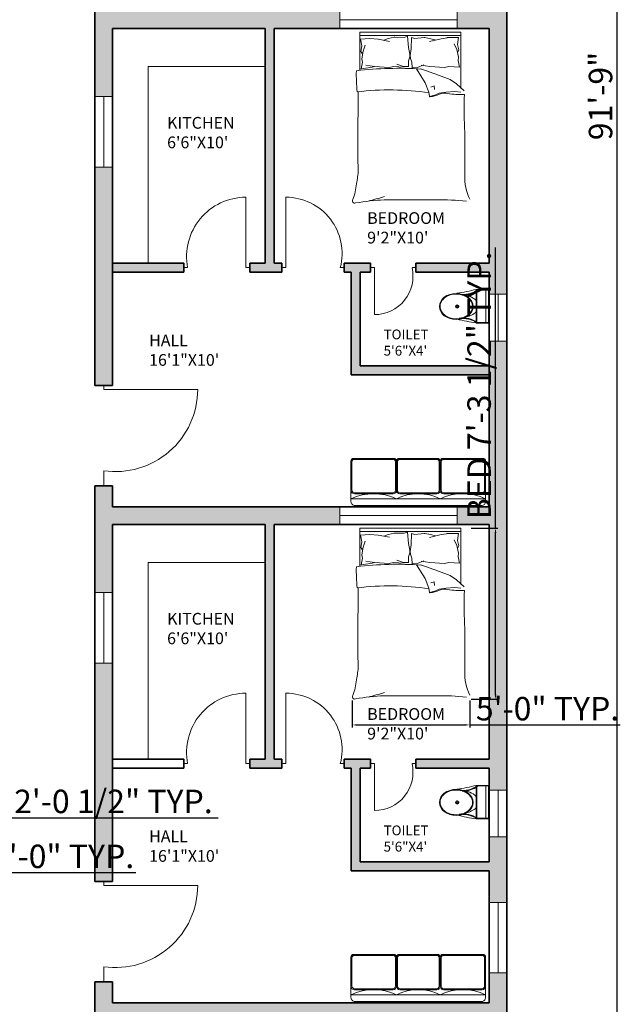
# Model space of a CAD drawing. Units: inches. Extents: x 1266 to 2869, y -408 to 3241.
# Tile 3 of 11: x 1710 to 2017, y 1264 to 1767. Entities that reach past the tile are written whole.
import ezdxf

# ---------------------------------------------------------------- set-up
doc = ezdxf.new("R2010")
doc.units = ezdxf.units.IN
for name, color, linetype, lineweight in [('A-ANNO-DIMS', 2, 'Continuous', 18), ('A-AREA-IDEN', 7, 'Continuous', 18), ('A-DOOR', 4, 'Continuous', 18), ('A-FLOR-CASE', 9, 'Continuous', 18), ('A-FLOR-FIXT', 9, 'Continuous', 18), ('A-FURN', 8, 'Continuous', 18), ('A-GLAZ', 4, 'Continuous', 18), ('A-WALL', 7, 'Continuous', 35), ('A-WALL-PATT', 251, 'Continuous', 13)]:
    doc.layers.add(name, color=color, linetype=linetype, lineweight=lineweight)
doc.styles.get("Standard").update_dxf_attribs({"font": 'arial.ttf'})
doc.dimstyles.new('ISO-25', dxfattribs={"dimtxt": 12, "dimasz": 2.5, "dimexe": 1.25, "dimexo": 0.625, "dimtad": 1, "dimdec": 0, "dimlunit": 3, "dimtxsty": 'Standard', "dimcen": 2.5, "dimadec": 0, "dimazin": 0, "dimtfac": 1, "dimtdec": 0, "dimtmove": 0, "dimatfit": 3, "dimfxl": 1, "dimarcsym": 0})

# ---------------------------------------------------------------- blocks, each defined once
blk = doc.blocks.new('A$C31115884')
for p, q in [((283, 498), (223, 498)), ((258, 466), (258, 523)), ((0, 200), (0, 0)), ((520, 200), (0, 200)), ((10, 190), (10, 10)), ((510, 190), (10, 190)), ((510, 10), (510, 190)), ((520, 0), (520, 200)), ((510, 54), (0, 54)), ((10, 10), (510, 10)), ((0, 0), (520, 0))]:
    blk.add_line(p, q)
blk.add_circle((256, 496), 23.6)
for centre, radius, start, end in [((2778, -205), 2807, 165.4549, 171.7133), ((-295, 403), 365, 324.2091, 9.3499), ((-295, 403), 375, 324.2091, 9.3499), ((806, 403), 365, 170.6501, 215.7909), ((3237, 905), 2807, 188.2867, 194.5451), ((384, 406), 293, 190.2774, 224.1564), ((139, 406), 293, 315.8436, 2.6563), ((806, 403), 375, 179.2036, 215.7909)]:
    blk.add_arc(centre, radius, start, end)
blk.add_ellipse((256, 510), major_axis=(0, -261), ratio=0.772727)
blk.add_open_spline([(256, 259), (263, 259), (270, 260), (288, 262), (299, 265), (320, 273), (330, 278), (350, 291), (360, 299), (378, 316), (386, 326), (402, 347), (409, 358), (421, 383), (427, 395), (436, 422), (440, 436), (445, 465), (447, 480), (448, 509), (448, 524), (445, 553), (443, 568), (436, 596), (432, 610), (422, 636), (416, 649), (402, 672), (395, 683), (379, 703), (370, 712), (351, 728), (341, 735), (321, 746), (310, 751), (289, 757), (278, 759), (256, 761), (245, 761), (223, 757), (212, 754), (191, 746), (181, 741), (161, 728), (151, 720), (133, 703), (125, 693), (110, 672), (103, 660), (90, 636), (85, 623), (76, 596), (72, 582), (67, 553), (66, 538), (64, 509), (65, 494), (68, 465), (70, 450), (77, 422), (81, 408), (91, 382), (97, 370), (111, 346), (118, 335), (135, 316), (144, 307), (162, 291), (172, 284), (193, 273), (203, 269), (225, 262), (236, 260), (250, 259), (253, 259), (256, 259)], degree=3, knots=[0, 0, 0, 0, 0.110105, 0.110105, 0.285049, 0.285049, 0.459994, 0.459994, 0.634938, 0.634938, 0.809882, 0.809882, 0.984827, 0.984827, 1.159771, 1.159771, 1.334715, 1.334715, 1.50966, 1.50966, 1.684604, 1.684604, 1.859549, 1.859549, 2.034493, 2.034493, 2.209437, 2.209437, 2.384382, 2.384382, 2.559326, 2.559326, 2.73427, 2.73427, 2.909215, 2.909215, 3.084159, 3.084159, 3.259103, 3.259103, 3.434048, 3.434048, 3.608992, 3.608992, 3.783936, 3.783936, 3.958881, 3.958881, 4.133825, 4.133825, 4.30877, 4.30877, 4.483714, 4.483714, 4.658658, 4.658658, 4.833603, 4.833603, 5.008547, 5.008547, 5.183491, 5.183491, 5.358436, 5.358436, 5.53338, 5.53338, 5.708324, 5.708324, 5.883269, 5.883269, 6.058213, 6.058213, 6.233158, 6.233158, 6.283185, 6.283185, 6.283185, 6.283185])
blk = doc.blocks.new('*D3')
at = {"layer": 'A-ANNO-DIMS', "color": 0, "lineweight": -2, "transparency": 16777216}
for p, q in [((1959.32, 2278.35), (2016.1, 2278.35)), ((2014.85, 2275.85), (2014.85, 1179.85)), ((1959.32, 1177.35), (2016.1, 1177.35))]:
    blk.add_line(p, q, dxfattribs=at)
at = {"layer": 'A-ANNO-DIMS', "color": 0, "transparency": 16777216}
for points in [[(2014.43, 2275.85), (2015.27, 2275.85), (2014.85, 2278.35)], [(2014.43, 1179.85), (2015.27, 1179.85), (2014.85, 1177.35)]]:
    blk.add_solid(points, dxfattribs=at)
at = {"layer": 'Defpoints', "color": 0, "transparency": 16777216}
for p in [(1958.69, 2278.35), (1958.69, 1177.35), (2014.85, 1177.35)]:
    blk.add_point(p, dxfattribs=at)
at = {"layer": 'A-ANNO-DIMS', "color": 0, "transparency": 16777216, "insert": (2008.1, 1727.85), "char_height": 12, "attachment_point": 5, "rotation": 90}
blk.add_mtext('91\'-9"', dxfattribs=at)
blk = doc.blocks.new('BED-DOUBLE-2')
for p, q in [((3.76, 67.77), (3.76, 87.35)), ((3.76, 87.35), (55.42, 87.35)), ((3.76, 85.69), (55.42, 85.69)), ((55.42, 87.35), (55.42, 58.59)), ((4.21, 83.74), (8.84, 84.1)), ((4.21, 83.77), (4.84, 80.33)), ((5.46, 77.67), (6.55, 80.64)), ((8.84, 84.1), (8.96, 84.08)), ((8.96, 84.08), (13.09, 83.77)), ((13.09, 83.77), (19.03, 82.67)), ((16.06, 83.3), (18.25, 84.08)), ((18.25, 84.08), (21.37, 84.86)), ((21.37, 84.86), (21.72, 84.86)), ((21.72, 84.86), (26.53, 84.7)), ((26.53, 84.7), (28.09, 85.33)), ((28.09, 85.33), (28.71, 79.55)), ((30.24, 84.66), (29.98, 78.85)), ((31.84, 84.13), (30.24, 84.66)), ((36.63, 84.59), (31.84, 84.13)), ((36.98, 84.61), (36.63, 84.59)), ((40.14, 84.02), (36.98, 84.61)), ((45.31, 84.03), (39.45, 82.57)), ((42.38, 83.38), (40.14, 84.02)), ((49.42, 84.6), (45.31, 84.03)), ((54.17, 84.59), (48.33, 84.69)), ((48.33, 84.69), (49.42, 84.6)), ((53.31, 78.43), (52.03, 81.32)), ((54.17, 84.59), (53.76, 81.12)), ((53.76, 81.12), (54.41, 78.34)), ((4.84, 80.33), (4.37, 77.51)), ((4.37, 77.51), (4.99, 76.42)), ((4.84, 73.76), (5.46, 77.67)), ((28.71, 79.55), (29.34, 76.11)), ((29.34, 76.11), (29.34, 74.7)), ((29.98, 78.85), (29.57, 75.38)), ((54.17, 74.56), (53.31, 78.43)), ((54.41, 78.34), (53.85, 77.21)), ((4.52, 68.61), (5.15, 72.04)), ((5.15, 72.04), (4.84, 73.76)), ((26.06, 69.77), (22.66, 70.95)), ((29.34, 74.7), (28.71, 72.67)), ((28.71, 72.67), (28.71, 69.77)), ((29.57, 75.38), (29.66, 73.97)), ((29.66, 73.97), (30.41, 71.98)), ((30.41, 71.98), (30.59, 69.09)), ((33.24, 69.26), (36.56, 70.64)), ((53.97, 72.83), (54.17, 74.56)), ((54.81, 69.44), (53.97, 72.83)), ((10.03, 69.39), (4.52, 68.61)), ((6.9, 70.46), (11.26, 69.74)), ((11.26, 69.74), (10.03, 69.39)), ((11.26, 69.74), (18.84, 69.27)), ((18.84, 69.27), (20.95, 69.87)), ((20.95, 69.87), (26.5, 69.44)), ((28.71, 69.77), (26.06, 69.77)), ((30.59, 69.09), (33.24, 69.26)), ((32.71, 68.56), (37.24, 61.54)), ((43.94, 65.39), (34.92, 68.56)), ((35.2, 70.46), (39.56, 69.74)), ((39.56, 69.74), (47.14, 69.27)), ((47.14, 69.27), (49.26, 69.87)), ((49.26, 69.87), (54.81, 69.44)), ((37.24, 61.54), (39.08, 56.69)), ((49.96, 63.21), (43.94, 65.39)), ((53.15, 60.87), (49.96, 63.21)), ((57.15, 57.36), (53.15, 60.87)), ((39.08, 56.69), (39.42, 54.51)), ((40.12, 59.32), (41.78, 59.99)), ((41.87, 58.1), (41.78, 59.99, 4.18)), ((42.1, 55.18), (44.27, 56.19)), ((44.27, 56.19), (47.96, 56.69)), ((47.96, 56.69), (52.14, 57.02)), ((52.14, 57.02), (55.49, 56.69)), ((39.42, 54.51), (42.1, 55.18)), ((16.28, 1.69), (42.89, 1.69))]:
    blk.add_line(p, q)
for centre, radius, start, end in [((92.06, 65.63), 90.06, 178.7218, 185.604), ((23.09, -109.45), 178.34, 86.0865, 96.7821), ((19.19, -81.63), 139.47, 81.7845, 96.9006), ((-180.86, 53.65), 183.89, 358.4762, 1.0082), ((33.68, 85.75), 32.06, 280.6617, 289.8806), ((47.29, 49.44), 6.73, 78.6608, 113.7384), ((55.49, 94.55), 39.11, 259.8763, 272.5657), ((197.03, 48.09), 139.99, 176.9791, 183.8365), ((39.61, 54.45), 0.199, 160.2464, 271.1377), ((524.11, 32.64), 521.39, 178.2277, 181.7185), ((-4874.07, 14.03), 4931.49, 0.00217, 0.28689), ((-29.08, 17.61), 32.04, 346.0648, 358.9113), ((82.33, 13.12), 24.93, 177.4714, 206.4681), ((-23.41, 11.38), 25.47, 337.9751, 356.652), ((1.18, 1.17), 1.18, 146.1736, 293.4781), ((23.16, -129.76), 131.62, 92.9958, 99.4091), ((-18.62, 112.98), 115.08, 283.3832, 287.7053), ((44.49, -142.12), 143.82, 84.4998, 90.6351)]:
    blk.add_arc(centre, radius, start, end)
blk = doc.blocks.new('SOFA-3-SEAT')
for points in [[(0, 22.36), (0, 7.74, 0.414214), (1.72, 6.02), (21.5, 6.02, 0.414214), (23.22, 7.74), (23.22, 22.36, 0.414214), (21.5, 24.08), (1.72, 24.08, 0.414214)], [(0.52, 22.36), (0.52, 7.74, 0.414214), (1.72, 6.54), (21.5, 6.54, 0.414214), (22.7, 7.74), (22.7, 22.36, 0.414214), (21.5, 23.56), (1.72, 23.56, 0.414214)], [(45.57, 22.36), (45.57, 7.74, -0.414214), (43.85, 6.02), (24.94, 6.02, -0.414214), (23.22, 7.74), (23.22, 22.36, -0.414214), (24.94, 24.08), (43.85, 24.08, -0.414214)], [(45.06, 22.36), (45.06, 7.74, -0.414214), (43.85, 6.54), (24.94, 6.54, -0.414214), (23.73, 7.74), (23.73, 22.36, -0.414214), (24.94, 23.56), (43.85, 23.56, -0.414214)], [(45.57, 22.36), (45.57, 7.74, 0.414214), (47.29, 6.02), (67.07, 6.02, 0.414214), (68.79, 7.74), (68.79, 22.36, 0.414214), (67.07, 24.08), (47.29, 24.08, 0.414214)], [(46.09, 22.36), (46.09, 7.74, 0.414214), (47.29, 6.54), (67.07, 6.54, 0.414214), (68.27, 7.74), (68.27, 22.36, 0.414214), (67.07, 23.56), (47.29, 23.56, 0.414214)]]:
    blk.add_lwpolyline(points, format="xyb", close=True)
at = {"ltscale": 0.03}
blk.add_lwpolyline([(21.82, 24.08), (1.38, 24.08, 0.414214), (0, 22.7), (0, 2.06, 0.414214), (2.06, 0), (66.73, 0, 0.414214), (68.79, 2.06), (68.79, 22.7, 0.414214), (67.41, 24.08), (46.97, 24.08, 0.414214), (45.59, 22.7, -1), (45.56, 22.7, 0.414214), (44.18, 24.08), (24.61, 24.08, 0.414214), (23.23, 22.7, -1), (23.2, 22.7, 0.414214)], format="xyb", close=True, dxfattribs=at)
blk.add_lwpolyline([(0, 3.44), (68.79, 3.44)])
for centre, radius, start, end in [((11.61, -21.35), 27.38, 64.9106, 115.0894), ((34.4, -19.35), 25.38, 63.869, 116.131), ((57.18, -21.07), 27.12, 64.6538, 115.3462)]:
    blk.add_arc(centre, radius, start, end)
blk = doc.blocks.new('DOOR-KITCHEN-R')
for p, q in [((31.78, 0), (31.78, 36)), ((0, 0), (2, 0)), ((33.78, 0), (31.78, 0))]:
    blk.add_line(p, q)
blk.add_arc((31.78, 5.68), 30.32, 90, 190.7956)
blk = doc.blocks.new('DOOR-BEDROOM-R')
for p, q in [((2, 0), (2, 36)), ((0, 0), (2, 0)), ((31.84, 0), (29.84, 0))]:
    blk.add_line(p, q)
blk.add_arc((2, 7.24), 28.76, 345.4318, 90)
blk = doc.blocks.new('DOOR-BATH-R')
for p, q in [((0, 24), (2, 24)), ((2, 24), (2, 0)), ((23.14, 24), (21.14, 24))]:
    blk.add_line(p, q)
blk.add_arc((2, 19.63), 19.63, 270, 12.8499)
blk = doc.blocks.new('DOOR-ENTRY-R')
for p, q in [((0, 51.27), (0, 49.27)), ((0, 49.27), (36, 49.27)), ((36, 49.27), (48, 49.27)), ((0, 5.68), (0, 7.68)), ((0, 0), (0, 5.68))]:
    blk.add_line(p, q)
blk.add_arc((5.98, 49.27), 42.02, 261.8116, 0)
blk = doc.blocks.new('WIN-PLAN-60')
for p, q in [((0, 9), (0, 0)), ((60, 4.5), (60, 9)), ((60, 9), (60, 0)), ((0, 4.5), (60, 4.5)), ((0, 0), (0, 4.5))]:
    blk.add_line(p, q)
blk = doc.blocks.new('WIN-PLAN-36')
for p, q in [((0, 36), (9, 36)), ((4.5, 36), (4.5, 0)), ((9, 36), (4.5, 36)), ((4.5, 0), (0, 0)), ((0, 0), (9, 0))]:
    blk.add_line(p, q)
blk = doc.blocks.new('WIN-PLAN-24')
for p, q in [((0, 24), (9, 24)), ((4.5, 24), (4.5, 0)), ((9, 24), (4.5, 24)), ((0, 0), (9, 0))]:
    blk.add_line(p, q)
blk = doc.blocks.new('COUNTER-KITCHEN')
for p, q in [((0, 0), (0, 100.54)), ((0, 100.54), (59.82, 100.54))]:
    blk.add_line(p, q)
blk = doc.blocks.new('*D35')
at = {"layer": 'A-ANNO-DIMS', "color": 0, "lineweight": -2, "transparency": 16777216}
for p, q in [((1627.24, 1361.97), (1627.24, 1357.64)), ((1629.74, 1358.89), (1649.44, 1358.89)), ((1651.94, 1361.97), (1651.94, 1357.64)), ((1651.94, 1358.89), (1811.15, 1358.89))]:
    blk.add_line(p, q, dxfattribs=at)
at = {"layer": 'A-ANNO-DIMS', "color": 0, "transparency": 16777216}
for points in [[(1629.74, 1359.31), (1629.74, 1358.48), (1627.24, 1358.89)], [(1649.44, 1359.31), (1649.44, 1358.48), (1651.94, 1358.89)]]:
    blk.add_solid(points, dxfattribs=at)
at = {"layer": 'Defpoints', "color": 0, "transparency": 16777216}
for p in [(1627.24, 1362.6), (1651.94, 1362.6), (1651.94, 1358.89)]:
    blk.add_point(p, dxfattribs=at)
at = {"layer": 'A-ANNO-DIMS', "color": 0, "transparency": 16777216, "insert": (1732.8, 1365.73), "char_height": 12, "attachment_point": 5}
blk.add_mtext('DOOR 2\'-0 1/2" TYP.', dxfattribs=at)
blk = doc.blocks.new('*D41')
at = {"layer": 'A-ANNO-DIMS', "color": 0, "lineweight": -2, "transparency": 16777216}
for p, q in [((1952.88, 1506.96), (1952.88, 1650.41)), ((1940.39, 1506.96), (1954.13, 1506.96)), ((1952.88, 1421.99), (1952.88, 1504.46)), ((1940.39, 1419.49), (1954.13, 1419.49))]:
    blk.add_line(p, q, dxfattribs=at)
at = {"layer": 'A-ANNO-DIMS', "color": 0, "transparency": 16777216}
for points in [[(1952.46, 1504.46), (1953.3, 1504.46), (1952.88, 1506.96)], [(1952.46, 1421.99), (1953.3, 1421.99), (1952.88, 1419.49)]]:
    blk.add_solid(points, dxfattribs=at)
at = {"layer": 'Defpoints', "color": 0, "transparency": 16777216}
for p in [(1939.76, 1506.96), (1952.88, 1506.96), (1939.76, 1419.49)]:
    blk.add_point(p, dxfattribs=at)
at = {"layer": 'A-ANNO-DIMS', "color": 0, "transparency": 16777216, "insert": (1946.05, 1579.94), "char_height": 12, "attachment_point": 5, "rotation": 90}
blk.add_mtext('BED 7\'-3 1/2" TYP.', dxfattribs=at)
blk = doc.blocks.new('*D42')
at = {"layer": 'A-ANNO-DIMS', "color": 0, "lineweight": -2, "transparency": 16777216}
for p, q in [((1879.66, 1418.87), (1879.66, 1405.12)), ((1939.76, 1418.87), (1939.76, 1405.12)), ((1882.16, 1406.37), (1937.26, 1406.37)), ((1939.76, 1406.37), (2016.66, 1406.37))]:
    blk.add_line(p, q, dxfattribs=at)
at = {"layer": 'A-ANNO-DIMS', "color": 0, "transparency": 16777216}
for points in [[(1882.16, 1406.79), (1882.16, 1405.96), (1879.66, 1406.37)], [(1937.26, 1406.79), (1937.26, 1405.96), (1939.76, 1406.37)]]:
    blk.add_solid(points, dxfattribs=at)
at = {"layer": 'Defpoints', "color": 0, "transparency": 16777216}
for p in [(1879.66, 1419.49), (1939.76, 1419.49), (1939.76, 1406.37)]:
    blk.add_point(p, dxfattribs=at)
at = {"layer": 'A-ANNO-DIMS', "color": 0, "transparency": 16777216, "insert": (1979.46, 1413.13), "char_height": 12, "attachment_point": 5}
blk.add_mtext('5\'-0" TYP.', dxfattribs=at)
blk = doc.blocks.new('*D46')
at = {"layer": 'A-ANNO-DIMS', "color": 0, "lineweight": -2, "transparency": 16777216}
for p, q in [((1643.69, 1323.83), (1643.69, 1332.15)), ((1646.19, 1330.9), (1689.19, 1330.9)), ((1691.69, 1323.83), (1691.69, 1332.15)), ((1691.69, 1330.9), (1769.07, 1330.9))]:
    blk.add_line(p, q, dxfattribs=at)
at = {"layer": 'A-ANNO-DIMS', "color": 0, "transparency": 16777216}
for points in [[(1646.19, 1331.32), (1646.19, 1330.48), (1643.69, 1330.9)], [(1689.19, 1331.32), (1689.19, 1330.48), (1691.69, 1330.9)]]:
    blk.add_solid(points, dxfattribs=at)
at = {"layer": 'Defpoints', "color": 0, "transparency": 16777216}
for p in [(1691.69, 1330.9), (1643.69, 1323.21), (1691.69, 1323.21)]:
    blk.add_point(p, dxfattribs=at)
at = {"layer": 'A-ANNO-DIMS', "color": 0, "transparency": 16777216, "insert": (1731.63, 1337.65), "char_height": 12, "attachment_point": 5}
blk.add_mtext('4\'-0" TYP.', dxfattribs=at)

msp = doc.modelspace()

# ---------------------------------------------------------------- hatches: boundary and pattern name
at = {"layer": 'A-WALL-PATT'}
h = msp.add_hatch(color=256, dxfattribs=at)
h.dxf.hatch_style = 1
h.paths.add_polyline_path([(1484.69, 2269.35), (1562.69, 2269.35), (1562.69, 2149.35), (1558.42, 2149.35), (1558.42, 2144.85), (1567.19, 2144.85), (1573.23, 2144.85), (1573.23, 2146.74), (1573.23, 2149.35), (1567.19, 2149.35), (1567.19, 2269.35), (1597.45, 2269.35), (1597.45, 2273.85), (1597.45, 2278.35), (1475.69, 2278.35), (1475.69, 2234.52), (1484.69, 2234.52)])
h.paths.add_polyline_path([(1873.25, 2278.35), (1748.19, 2278.35), (1696.19, 2278.35), (1657.45, 2278.35), (1657.45, 2269.35), (1687.19, 2269.35), (1687.19, 2149.35), (1651.94, 2149.35), (1651.94, 2144.85), (1687.19, 2144.85), (1687.19, 2133.61), (1696.19, 2133.61), (1696.19, 2269.35), (1748.19, 2269.35), (1748.19, 2234.52), (1757.19, 2234.52), (1757.19, 2269.35), (1835.19, 2269.35), (1835.19, 2149.35), (1827.33, 2149.35), (1827.33, 2144.85), (1843.74, 2144.85), (1843.74, 2149.35), (1839.69, 2149.35), (1839.69, 2269.35), (1873.25, 2269.35), (1873.25, 2273.85)])
h.paths.add_polyline_path([(1958.69, 2278.35), (1933.25, 2278.35), (1933.25, 2269.35), (1949.69, 2269.35), (1949.69, 2149.35), (1912.22, 2149.35), (1912.22, 2144.85), (1949.69, 2144.85), (1949.69, 2133.61), (1958.69, 2133.61)])
h.paths.add_polyline_path([(1883.69, 2144.85), (1889.08, 2144.85), (1889.08, 2149.35), (1875.58, 2149.35), (1875.58, 2144.85), (1879.19, 2144.85), (1879.19, 2092.35), (1949.69, 2092.35), (1949.69, 2086.89), (1949.69, 2024.85), (1933.25, 2024.85), (1933.25, 2015.85), (1949.69, 2015.85), (1949.69, 1895.85), (1912.45, 1895.85), (1912.45, 1891.35), (1949.69, 1891.35), (1949.69, 1880.11), (1958.69, 1880.11), (1958.69, 2086.89), (1958.69, 2109.61), (1949.69, 2109.61), (1949.69, 2096.85), (1883.69, 2096.85)])
h.paths.add_polyline_path([(1757.19, 2198.52), (1748.19, 2198.52), (1748.19, 2086.89), (1757.19, 2086.89), (1757.19, 2144.85), (1793.55, 2144.85), (1793.55, 2149.35), (1757.19, 2149.35)])
h.paths.add_polyline_path([(1696.19, 2109.61), (1687.19, 2109.61), (1687.19, 2096.85), (1621.19, 2096.85), (1621.19, 2144.85), (1627.24, 2144.85), (1627.24, 2149.35), (1616.69, 2149.35), (1610.35, 2149.35), (1610.35, 2144.85), (1616.69, 2144.85), (1616.69, 2092.35), (1687.19, 2092.35), (1687.19, 2086.89), (1696.19, 2086.89)], flags=17)
h.paths.add_polyline_path([(1484.69, 2144.85), (1520.8, 2144.85), (1520.8, 2149.35), (1484.69, 2149.35), (1484.69, 2198.52), (1475.69, 2198.52), (1475.69, 1981.02), (1484.69, 1981.02), (1484.69, 2015.85), (1687.19, 2015.85), (1687.19, 1895.85), (1650.13, 1895.85), (1650.13, 1891.35), (1687.19, 1891.35), (1687.19, 1880.11), (1696.19, 1880.11), (1696.19, 2035.62), (1687.19, 2035.62), (1687.19, 2024.85), (1484.69, 2024.85)])
h.paths.add_polyline_path([(1484.69, 1691.52), (1475.69, 1691.52), (1475.69, 1474.02), (1484.69, 1474.02)])
h.paths.add_polyline_path([(1518.03, 1895.85), (1484.69, 1895.85), (1484.69, 1945.02), (1475.69, 1945.02), (1475.69, 1727.52), (1484.69, 1727.52), (1484.69, 1762.35), (1687.19, 1762.35), (1687.19, 1642.35), (1651.94, 1642.35), (1651.94, 1637.85), (1687.19, 1637.85), (1687.19, 1589.85), (1621.19, 1589.85), (1621.19, 1637.85), (1627.19, 1637.85), (1627.19, 1642.35), (1610.89, 1642.35), (1610.89, 1637.85), (1616.69, 1637.85), (1616.69, 1585.35), (1687.19, 1585.35), (1687.19, 1579.45), (1696.19, 1579.45), (1696.19, 1779.84), (1687.19, 1779.84), (1687.19, 1771.35), (1484.69, 1771.35), (1484.69, 1891.35), (1518.03, 1891.35)])
h.paths.add_polyline_path([(1567.19, 2015.85), (1562.69, 2015.85), (1562.69, 1895.85), (1555.64, 1895.85), (1555.64, 1891.35), (1570.46, 1891.35), (1570.46, 1895.85), (1567.19, 1895.85)], flags=17)
h.paths.add_polyline_path([(1625.43, 1895.85), (1607.58, 1895.85), (1607.58, 1891.35), (1616.69, 1891.35), (1616.69, 1838.85), (1687.19, 1838.85), (1687.19, 1831.11), (1696.19, 1831.11), (1696.19, 1856.11), (1687.19, 1856.11), (1687.19, 1843.35), (1621.19, 1843.35), (1621.19, 1891.35), (1625.43, 1891.35)], flags=17)
h.paths.add_polyline_path([(1567.19, 1762.35), (1562.69, 1762.35), (1562.69, 1642.35), (1558.42, 1642.35), (1558.42, 1637.85), (1573.23, 1637.85), (1573.23, 1642.35), (1567.19, 1642.35)], flags=17)
h.paths.add_polyline_path([(1520.8, 1642.35), (1484.69, 1642.35), (1484.69, 1637.85), (1520.8, 1637.85)], flags=17)
h.paths.add_polyline_path([(1687.19, 1517.85), (1484.69, 1517.85), (1484.69, 1508.85), (1562.69, 1508.85), (1562.69, 1388.85), (1567.19, 1388.85), (1567.19, 1508.85), (1687.19, 1508.85)])
h.paths.add_polyline_path([(1696.19, 1528.18), (1687.19, 1528.18), (1687.19, 1323.21), (1696.19, 1323.21)])
h.paths.add_polyline_path([(1696.19, 1271.94), (1687.19, 1271.94), (1687.19, 1264.35), (1484.69, 1264.35), (1484.69, 1283.77), (1480.19, 1283.77), (1475.69, 1283.77), (1475.69, 1255.35), (1480.19, 1255.35), (1696.19, 1255.35)])
h.paths.add_polyline_path([(1484.69, 1438.02), (1475.69, 1438.02), (1475.69, 1319.77), (1484.69, 1319.77)])
h.paths.add_polyline_path([(1873.25, 1513.35), (1873.25, 1517.85), (1757.19, 1517.85), (1757.19, 1528.62), (1748.19, 1528.62), (1748.19, 1474.02), (1757.19, 1474.02), (1757.19, 1508.85), (1835.19, 1508.85), (1835.19, 1388.85), (1827.33, 1388.85), (1827.33, 1384.35), (1843.74, 1384.35), (1843.74, 1388.85), (1839.69, 1388.85), (1839.69, 1508.85), (1873.25, 1508.85)])
h.paths.add_polyline_path([(1958.69, 1602.61), (1949.69, 1602.61), (1949.69, 1517.85), (1933.25, 1517.85), (1933.25, 1508.85), (1949.69, 1508.85), (1949.69, 1388.85), (1912.22, 1388.85), (1912.22, 1384.35), (1949.69, 1384.35), (1949.69, 1373.11), (1958.69, 1373.11)])
h.paths.add_polyline_path([(1958.69, 1349.11), (1949.69, 1349.11), (1949.69, 1336.35), (1883.69, 1336.35), (1883.69, 1384.35), (1889.08, 1384.35), (1889.08, 1388.85), (1875.58, 1388.85), (1875.58, 1384.35), (1879.19, 1384.35), (1879.19, 1331.85), (1949.69, 1331.85), (1949.69, 1315.59), (1958.69, 1315.59)])
h.paths.add_polyline_path([(1958.69, 1279.59), (1954.19, 1279.59), (1949.69, 1279.59), (1949.69, 1264.35), (1757.19, 1264.35), (1757.19, 1275.12), (1748.19, 1275.12), (1748.19, 1255.35), (1958.69, 1255.35)])
h.paths.add_polyline_path([(1757.19, 1438.02), (1748.19, 1438.02), (1748.19, 1326.39), (1757.19, 1326.39)])
h.paths.add_polyline_path([(1793.55, 1388.85), (1757.19, 1388.85), (1757.19, 1384.35), (1793.55, 1384.35)], flags=0)
h = msp.add_hatch(color=256, dxfattribs=at)
h.dxf.hatch_style = 1
h.paths.add_polyline_path([(1873.25, 2020.35), (1873.25, 2024.85), (1757.19, 2024.85), (1757.19, 2035.62), (1748.19, 2035.62), (1748.19, 1981.02), (1757.19, 1981.02), (1757.19, 2015.85), (1835.19, 2015.85), (1835.19, 1895.85), (1827.57, 1895.85), (1827.57, 1891.35), (1843.96, 1891.35), (1843.96, 1895.85), (1839.69, 1895.85), (1839.69, 2015.85), (1873.25, 2015.85)])
h.paths.add_polyline_path([(1757.19, 1945.02), (1748.19, 1945.02), (1748.19, 1833.39), (1757.19, 1833.39), (1757.19, 1891.35), (1793.77, 1891.35), (1793.77, 1895.85), (1757.19, 1895.85)])
h.paths.add_polyline_path([(1873.25, 1771.35), (1757.19, 1771.35), (1757.19, 1787.8), (1748.19, 1787.8), (1748.19, 1727.52), (1757.19, 1727.52), (1757.19, 1762.35), (1835.19, 1762.35), (1835.19, 1642.35), (1827.33, 1642.35), (1827.33, 1637.85), (1843.74, 1637.85), (1843.74, 1642.35), (1839.69, 1642.35), (1839.69, 1762.35), (1873.25, 1762.35), (1873.25, 1766.85)])
h.paths.add_polyline_path([(1883.69, 1637.85), (1889.08, 1637.85), (1889.08, 1642.35), (1875.58, 1642.35), (1875.58, 1637.85), (1879.19, 1637.85), (1879.19, 1585.35), (1949.69, 1585.35), (1949.69, 1589.85), (1883.69, 1589.85)])
h.paths.add_polyline_path([(1958.69, 1856.11), (1949.69, 1856.11), (1949.69, 1843.35), (1883.69, 1843.35), (1883.69, 1891.35), (1889.31, 1891.35), (1889.31, 1895.85), (1875.8, 1895.85), (1875.8, 1891.35), (1879.19, 1891.35), (1879.19, 1838.85), (1949.69, 1838.85), (1949.69, 1771.35), (1933.25, 1771.35), (1933.25, 1762.35), (1949.69, 1762.35), (1949.69, 1642.35), (1912.22, 1642.35), (1912.22, 1637.85), (1949.69, 1637.85), (1949.69, 1626.61), (1958.69, 1626.61)])
h.paths.add_polyline_path([(1757.19, 1691.52), (1748.19, 1691.52), (1748.19, 1579.89), (1757.19, 1579.89)])
h.paths.add_polyline_path([(1793.55, 1642.35), (1757.19, 1642.35), (1757.19, 1637.85), (1793.55, 1637.85)], flags=17)

# ---------------------------------------------------------------- linework, layer by layer
at = {"layer": 'A-FURN'}
for points in [[(1879.02, 1540.88), (1879.02, 1526.26, 0.414214), (1880.74, 1524.54), (1900.51, 1524.54, 0.414214), (1902.23, 1526.26), (1902.23, 1540.88, 0.414214), (1900.51, 1542.6), (1880.74, 1542.6, 0.414214)], [(1879.53, 1540.88), (1879.53, 1526.26, 0.414214), (1880.74, 1525.06), (1900.51, 1525.06, 0.414214), (1901.72, 1526.26), (1901.72, 1540.88, 0.414214), (1900.51, 1542.09), (1880.74, 1542.09, 0.414214)], [(1924.59, 1540.88), (1924.59, 1526.26, -0.414214), (1922.87, 1524.54), (1903.95, 1524.54, -0.414214), (1902.23, 1526.26), (1902.23, 1540.88, -0.414214), (1903.95, 1542.6), (1922.87, 1542.6, -0.414214)], [(1924.07, 1540.88), (1924.07, 1526.26, -0.414214), (1922.87, 1525.06), (1903.95, 1525.06, -0.414214), (1902.75, 1526.26), (1902.75, 1540.88, -0.414214), (1903.95, 1542.09), (1922.87, 1542.09, -0.414214)], [(1924.59, 1540.88), (1924.59, 1526.26, 0.414214), (1926.31, 1524.54), (1946.09, 1524.54, 0.414214), (1947.81, 1526.26), (1947.81, 1540.88, 0.414214), (1946.09, 1542.6), (1926.31, 1542.6, 0.414214)], [(1925.11, 1540.88), (1925.11, 1526.26, 0.414214), (1926.31, 1525.06), (1946.09, 1525.06, 0.414214), (1947.29, 1526.26), (1947.29, 1540.88, 0.414214), (1946.09, 1542.09), (1926.31, 1542.09, 0.414214)]]:
    msp.add_lwpolyline(points, format="xyb", close=True, dxfattribs=at)
at = {"layer": 'A-FURN', "ltscale": 0.03}
msp.add_lwpolyline([(1900.84, 1542.6), (1880.39, 1542.6, 0.414214), (1879.02, 1541.23), (1879.02, 1520.59, 0.414214), (1881.08, 1518.53), (1945.74, 1518.53, 0.414214), (1947.81, 1520.59), (1947.81, 1541.23, 0.414214), (1946.43, 1542.6), (1925.98, 1542.6, 0.414214), (1924.61, 1541.23, -1), (1924.57, 1541.23, 0.414214), (1923.2, 1542.6), (1903.63, 1542.6, 0.414214), (1902.25, 1541.23, -1), (1902.22, 1541.23, 0.414214)], format="xyb", close=True, dxfattribs=at)
at = {"layer": 'A-FURN'}
msp.add_lwpolyline([(1879.02, 1521.97), (1947.81, 1521.97)], dxfattribs=at)
for centre, radius, start, end in [((1890.62, 1497.17), 27.38, 64.9106, 115.0894), ((1913.41, 1499.18), 25.38, 63.869, 116.131), ((1936.2, 1497.46), 27.12, 64.6538, 115.3462)]:
    msp.add_arc(centre, radius, start, end, dxfattribs=at)
at = {"layer": 'A-WALL'}
for p, q in [((1958.69, 1255.35), (1958.69, 2086.89)), ((1748.19, 1787.8), (1748.19, 1579.89)), ((1757.19, 1762.35), (1835.19, 1762.35)), ((1757.19, 1762.35), (1757.19, 1579.89)), ((1835.19, 1762.35), (1835.19, 1642.35)), ((1839.69, 1762.35), (1839.69, 1642.35)), ((1839.69, 1762.35), (1949.69, 1762.35)), ((1949.69, 1762.35), (1949.69, 1642.35)), ((1757.19, 1642.35), (1793.55, 1642.35)), ((1793.55, 1640.1), (1793.55, 1642.35)), ((1793.55, 1642.35), (1793.55, 1637.85)), ((1827.33, 1640.1), (1827.33, 1642.35)), ((1827.33, 1642.35), (1827.33, 1637.85)), ((1827.33, 1642.35), (1835.19, 1642.35)), ((1839.69, 1642.35), (1843.74, 1642.35)), ((1843.74, 1640.1), (1843.74, 1642.35)), ((1843.74, 1642.35), (1843.74, 1637.85)), ((1875.58, 1640.1), (1875.58, 1642.35)), ((1875.58, 1642.35), (1875.58, 1637.85)), ((1875.58, 1642.35), (1889.08, 1642.35)), ((1889.08, 1640.1), (1889.08, 1642.35)), ((1889.08, 1642.35), (1889.08, 1637.85)), ((1912.22, 1640.1), (1912.22, 1642.35)), ((1912.22, 1642.35), (1912.22, 1637.85)), ((1912.22, 1642.35), (1949.69, 1642.35)), ((1757.19, 1637.85), (1793.55, 1637.85)), ((1827.33, 1637.85), (1843.74, 1637.85)), ((1875.58, 1637.85), (1879.19, 1637.85)), ((1879.19, 1637.85), (1879.19, 1585.35)), ((1883.69, 1637.85), (1883.69, 1589.85)), ((1883.69, 1637.85), (1889.08, 1637.85)), ((1912.22, 1637.85), (1949.69, 1637.85)), ((1949.69, 1637.85), (1949.69, 1517.85)), ((1879.19, 1585.35), (1949.69, 1585.35)), ((1883.69, 1589.85), (1949.69, 1589.85)), ((1752.69, 1579.89), (1748.19, 1579.89)), ((1748.19, 1579.89), (1757.19, 1579.89)), ((1752.69, 1528.62), (1748.19, 1528.62)), ((1748.19, 1528.62), (1748.19, 1528.62)), ((1748.19, 1528.62), (1757.19, 1528.62)), ((1748.19, 1528.62), (1748.19, 1326.39)), ((1757.19, 1528.62), (1757.19, 1517.85)), ((1757.19, 1517.85), (1949.69, 1517.85)), ((1757.19, 1508.85), (1835.19, 1508.85)), ((1757.19, 1508.85), (1757.19, 1326.39)), ((1835.19, 1508.85), (1835.19, 1388.85)), ((1839.69, 1508.85), (1839.69, 1388.85)), ((1839.69, 1508.85), (1949.69, 1508.85)), ((1949.69, 1508.85), (1949.69, 1388.85)), ((1757.19, 1388.85), (1793.55, 1388.85)), ((1757.19, 1384.35), (1793.55, 1384.35)), ((1793.55, 1386.6), (1793.55, 1388.85)), ((1793.55, 1388.85), (1793.55, 1384.35)), ((1827.33, 1386.6), (1827.33, 1388.85)), ((1827.33, 1388.85), (1827.33, 1384.35)), ((1827.33, 1388.85), (1835.19, 1388.85)), ((1827.33, 1384.35), (1843.74, 1384.35)), ((1839.69, 1388.85), (1843.74, 1388.85)), ((1843.74, 1386.6), (1843.74, 1388.85)), ((1843.74, 1388.85), (1843.74, 1384.35)), ((1875.58, 1386.6), (1875.58, 1388.85)), ((1875.58, 1388.85), (1875.58, 1384.35)), ((1875.58, 1388.85), (1889.08, 1388.85)), ((1875.58, 1384.35), (1879.19, 1384.35)), ((1879.19, 1384.35), (1879.19, 1331.85)), ((1883.69, 1384.35), (1883.69, 1336.35)), ((1883.69, 1384.35), (1889.08, 1384.35)), ((1889.08, 1386.6), (1889.08, 1388.85)), ((1889.08, 1388.85), (1889.08, 1384.35)), ((1912.22, 1386.6), (1912.22, 1388.85)), ((1912.22, 1388.85), (1912.22, 1384.35)), ((1912.22, 1388.85), (1949.69, 1388.85)), ((1912.22, 1384.35), (1949.69, 1384.35)), ((1949.69, 1384.35), (1949.69, 1336.35)), ((1883.69, 1336.35), (1949.69, 1336.35)), ((1879.19, 1331.85), (1949.69, 1331.85)), ((1949.69, 1331.85), (1949.69, 1264.35)), ((1752.69, 1326.39), (1748.19, 1326.39)), ((1748.19, 1326.39), (1757.19, 1326.39)), ((1752.69, 1275.12), (1748.19, 1275.12)), ((1748.19, 1275.12), (1757.19, 1275.12)), ((1748.19, 1275.12), (1748.19, 1255.35)), ((1757.19, 1275.12), (1757.19, 1264.35)), ((1757.19, 1264.35), (1949.69, 1264.35))]:
    msp.add_line(p, q, dxfattribs=at)

# ---------------------------------------------------------------- block references
at = {"layer": 'A-DOOR'}
for name, p in [('DOOR-KITCHEN-R', (1793.55, 1640.1)), ('DOOR-BEDROOM-R', (1843.73, 1640.1)), ('DOOR-BATH-R', (1889.08, 1616.1)), ('DOOR-ENTRY-R', (1752.69, 1528.62)), ('DOOR-KITCHEN-R', (1793.55, 1386.6)), ('DOOR-BEDROOM-R', (1843.73, 1386.6)), ('DOOR-BATH-R', (1889.08, 1362.6)), ('DOOR-ENTRY-R', (1752.69, 1275.12))]:
    msp.add_blockref(name, p, dxfattribs=at)
at = {"layer": 'A-FLOR-CASE'}
for p in [(1775.37, 1642.35), (1775.37, 1388.85)]:
    msp.add_blockref('COUNTER-KITCHEN', p, dxfattribs=at)
at = {"layer": 'A-FLOR-FIXT', "xscale": 0.0330640103915726, "yscale": 0.0330640103915726, "zscale": 0.0330640103915726, "rotation": 89.99999999999996}
for p in [(1949.69, 1611.81), (1949.69, 1358.31)]:
    msp.add_blockref('A$C31115884', p, dxfattribs=at)
at = {"layer": 'A-FURN'}
for name, p in [('BED-DOUBLE-2', (1879.75, 1673.11)), ('BED-DOUBLE-2', (1879.75, 1419.61)), ('SOFA-3-SEAT', (1879.02, 1265.03))]:
    msp.add_blockref(name, p, dxfattribs=at)
at = {"layer": 'A-GLAZ'}
for name, p in [('WIN-PLAN-60', (1873.25, 1762.35)), ('WIN-PLAN-36', (1748.19, 1691.52)), ('WIN-PLAN-24', (1949.69, 1602.61)), ('WIN-PLAN-60', (1873.25, 1508.85)), ('WIN-PLAN-36', (1748.19, 1438.02)), ('WIN-PLAN-24', (1949.69, 1349.11))]:
    msp.add_blockref(name, p, dxfattribs=at)
at = {"layer": 'A-GLAZ', "rotation": 180}
msp.add_blockref('WIN-PLAN-36', (1958.69, 1315.59), dxfattribs=at)

# ---------------------------------------------------------------- texts
at = {"layer": 'A-AREA-IDEN', "attachment_point": 1}
for s, width, insert, char_height in [('KITCHEN\\P6\'6"X10\'', 112.1355, (1785.05, 1717.14), 6), ('BEDROOM\\P9\'2"X10\'', 62.026, (1887.3, 1668.46), 6), ('HALL\\P16\'1"X10\'', 100.9767, (1775.86, 1605.93), 6), ('TOILET\\P5\'6"X4\'', 46.3569, (1895.7, 1608.49), 5), ('KITCHEN\\P6\'6"X10\'', 112.1355, (1785.05, 1463.64), 6), ('BEDROOM\\P9\'2"X10\'', 62.026, (1887.3, 1414.96), 6), ('TOILET\\P5\'6"X4\'', 46.3569, (1895.7, 1354.99), 5), ('HALL\\P16\'1"X10\'', 100.9767, (1775.86, 1352.43), 6)]:
    msp.add_mtext_dynamic_manual_height_columns(s, width=width, gutter_width=12.5, heights=[0], dxfattribs=dict(at, insert=insert, char_height=char_height))

# ---------------------------------------------------------------- dimensions: what is measured, and where the dimension line sits
at = {"layer": 'A-ANNO-DIMS'}
dim = msp.add_linear_dim(base=(2014.85, 1177.35), p1=(1958.69, 2278.35), p2=(1958.69, 1177.35), angle=90, dimstyle='ISO-25', override={"dimclrd": 0, "dimclre": 0, "dimclrt": 0}, dxfattribs=at)
dim.commit()
dim.dimension.update_dxf_attribs({"geometry": '*D3', "text_midpoint": (2008.1, 1727.85)})
dim = msp.add_linear_dim(base=(1952.88, 1506.96), p1=(1939.76, 1419.49), p2=(1939.76, 1506.96), angle=90, text='BED <> TYP.', dimstyle='ISO-25', override={"dimdec": 1, "dimlfac": 1, "dimrnd": 0, "dimzin": 1, "dimdsep": 46, "dimlunit": 4, "dimfrac": 2}, dxfattribs=at)
dim.commit()
dim.dimension.update_dxf_attribs({"geometry": '*D41', "text_midpoint": (1946.05, 1579.94)})
for base, p1, p2, text, picture, middle in [((1939.76, 1406.37), (1879.66, 1419.49), (1939.76, 1419.49), '<> TYP.', '*D42', (1979.46, 1413.13)), ((1651.94, 1358.89), (1627.24, 1362.6), (1651.94, 1362.6), 'DOOR <> TYP.', '*D35', (1732.8, 1365.73)), ((1691.69, 1330.9), (1643.69, 1323.21), (1691.69, 1323.21), '<> TYP.', '*D46', (1731.63, 1337.65))]:
    dim = msp.add_linear_dim(base=base, p1=p1, p2=p2, text=text, dimstyle='ISO-25', override={"dimdec": 1, "dimlfac": 1, "dimrnd": 0, "dimzin": 1, "dimdsep": 46, "dimlunit": 4, "dimfrac": 2}, dxfattribs=at)
    dim.commit()
    dim.dimension.update_dxf_attribs({"geometry": picture, "text_midpoint": middle})

doc.saveas('drawing.dxf')
